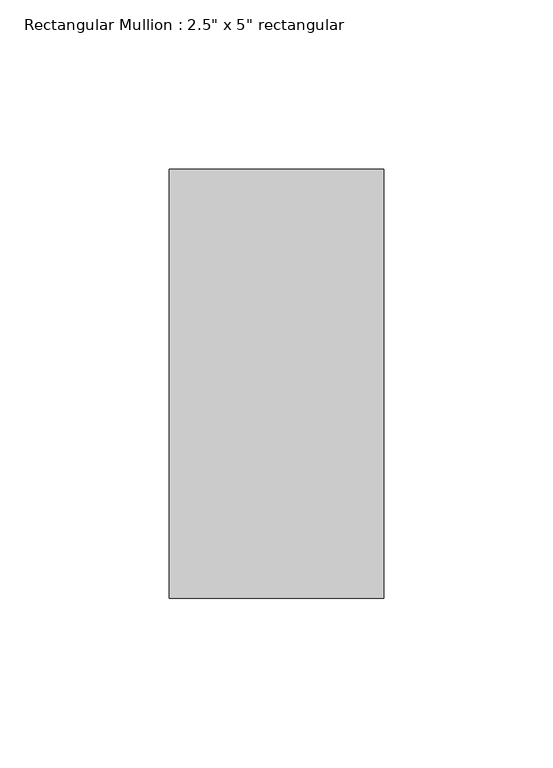
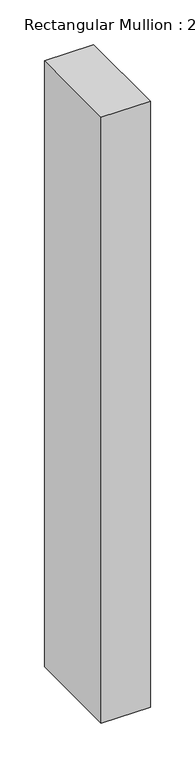
"""IFC4 building model written with IfcOpenShell, lengths in millimetres: member geometry."""

from ifc_helpers import new_model, si_unit, frame, origin, place, context, project, spatial, polyline, outline, extrude, source, transform, mapped, element, save


def member_0c7d0587(model_context):
    return source(origin(), model_context, "Body", "SweptSolid", [
        extrude(outline(polyline([(31.75, 63.5), (31.75, -63.5), (-31.75, -63.5), (-31.75, 63.5), (31.75, 63.5)])), frame((0.0, 0.0, -827.3309713), z_axis=(0.0, 0.0, 1.0), x_axis=(1.0, 0.0, 0.0)), (0.0, 0.0, 1.0), 827.3309713),
    ])


if __name__ == "__main__":
    model = new_model("IFC4")
    model_context = context("Model", 3, world=origin())
    ifc_project = project(units=[si_unit("LENGTHUNIT", "METRE", prefix="MILLI")], contexts=[model_context])
    site = spatial("IfcSite", under=ifc_project)
    building = spatial("IfcBuilding", under=site)
    placement = place(None, origin())
    member_shape = member_0c7d0587(model_context)
    element("IfcMember", 1, ObjectType="Rectangular Mullion : 2.5\" x 5\" rectangular", at=placement, inside=building, context=model_context, shape_type="MappedRepresentation", body=[
        mapped(member_shape, transform((0.0, 0.0, 0.0), x_axis=(1.0, 0.0, 0.0), y_axis=(0.0, 1.0, 0.0), z_axis=(0.0, 0.0, 1.0))),
    ])
    save(model, "model.ifc")

# Revit data of these elements
# Type "Rectangular Mullion : 2.5\" x 5\" rectangular"
#   built-in parameter 1007304 = 0.416667 (stored number, unit not read)
#   built-in parameter 1007301 = 0.104167 (stored number, unit not read)
#   built-in parameter 1007300 = 0.104167 (stored number, unit not read)
# Element 1 (IfcMember, "Rectangular Mullion : 2.5\" x 5\" rectangular")
#   Materials on its faces: "Aluminum"
# Materials
#   "Aluminum": class "Metal", colour RGB 247 247 247, transparency 0, Description = "Aluminum 6061", Cost = 0
